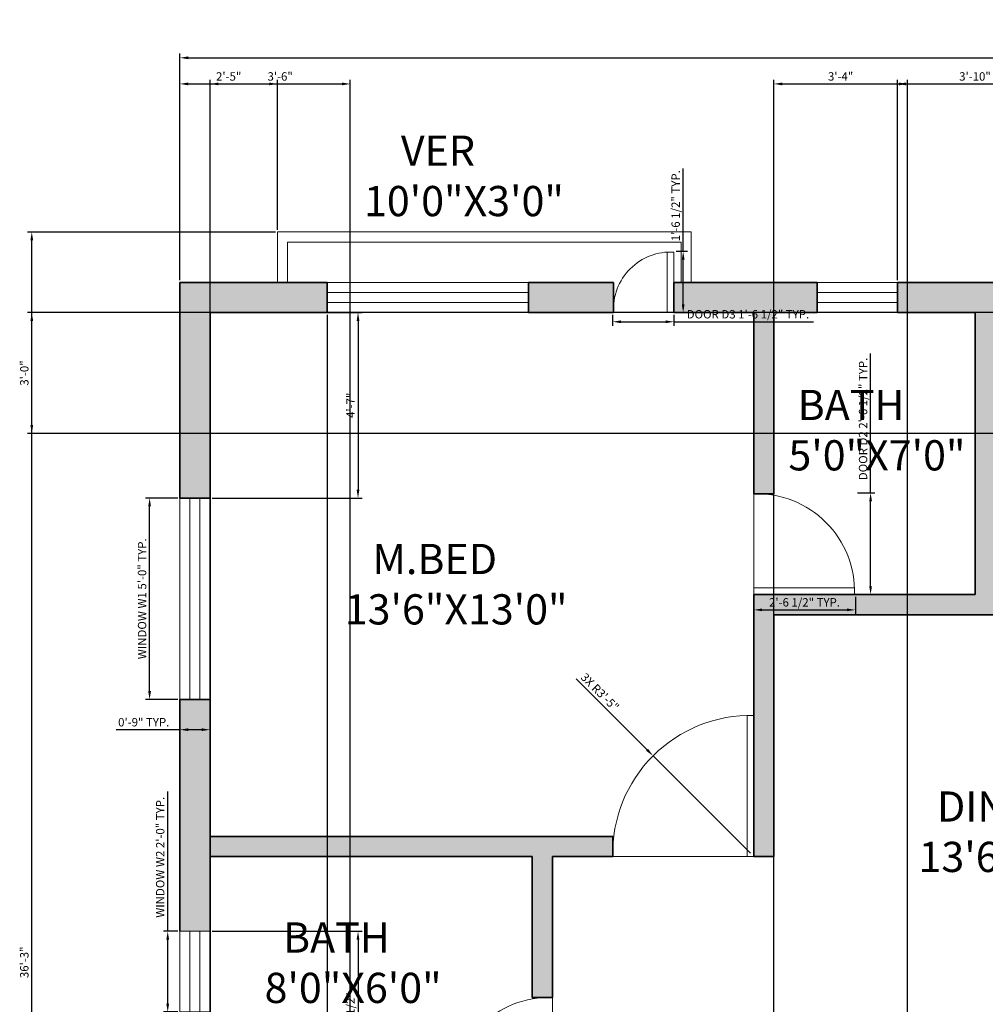
# Model space of a CAD drawing. Units: inches. Extents: x 1851 to 3979, y 3948 to 8145.
# Tile 2 of 4: x 1851 to 2139, y 4198 to 4491. Entities that reach past the tile are written whole.
import ezdxf

# ---------------------------------------------------------------- set-up
doc = ezdxf.new("R2010")
doc.units = ezdxf.units.IN
for name, color, linetype, lineweight in [('A-ANNO-DIMS', 2, 'Continuous', 18), ('A-GLAZ', 140, 'Continuous', 18), ('A-WALL', 7, 'Continuous', 35)]:
    doc.layers.add(name, color=color, linetype=linetype, lineweight=lineweight)
for name, color, linetype, lineweight, true_color in [('A-AREA-IDEN', 9, 'Continuous', 18, 0xc7c8ca), ('A-DOOR', 52, 'Continuous', 18, 0xc8c92d), ('A-FLOR-RAIL', 52, 'Continuous', 18, 0xc8c92d), ('A-WALL-PATT', 159, 'Continuous', 13, 0x22346e)]:
    doc.layers.add(name, color=color, linetype=linetype, lineweight=lineweight, true_color=true_color)
doc.styles.get("Standard").update_dxf_attribs({"font": 'arial.ttf'})
doc.dimstyles.new('ISO-25', dxfattribs={"dimtxt": 2.5, "dimasz": 2.5, "dimexe": 1.25, "dimexo": 0.625, "dimtad": 1, "dimlunit": 3, "dimtxsty": 'Standard', "dimcen": 2.5, "dimadec": 0, "dimazin": 0, "dimtfac": 1, "dimtmove": 0, "dimatfit": 3, "dimfxl": 1, "dimarcsym": 0})

# ---------------------------------------------------------------- blocks, each defined once
blk = doc.blocks.new('*D1')
at = {"layer": 'A-ANNO-DIMS', "color": 0, "lineweight": -2, "transparency": 16777216}
for p, q in [((1898.74, 4438.02), (1898.74, 4480.98)), ((2677.74, 4438.02), (2677.74, 4480.98)), ((1901.24, 4479.73), (2675.24, 4479.73))]:
    blk.add_line(p, q, dxfattribs=at)
at = {"layer": 'A-ANNO-DIMS', "color": 0, "transparency": 16777216}
for points in [[(1901.24, 4480.15), (1901.24, 4479.31), (1898.74, 4479.73)], [(2675.24, 4480.15), (2675.24, 4479.31), (2677.74, 4479.73)]]:
    blk.add_solid(points, dxfattribs=at)
at = {"layer": 'Defpoints', "color": 0, "transparency": 16777216}
for p in [(2677.74, 4479.73), (1898.74, 4437.39), (2677.74, 4437.39)]:
    blk.add_point(p, dxfattribs=at)
at = {"layer": 'A-ANNO-DIMS', "color": 0, "transparency": 16777216, "insert": (2288.24, 4484.95), "char_height": 9, "attachment_point": 5}
blk.add_mtext('64\'-11"', dxfattribs=at)
blk = doc.blocks.new('DOOR-SINGLE-42IN')
for p, q in [((42, 42), (40, 42)), ((40, 42), (40, 0)), ((42, 0), (42, 42)), ((40, 0), (42, 0))]:
    blk.add_line(p, q)
blk.add_arc((41, 1), 41.01, 88.6028, 181.3972)
blk = doc.blocks.new('DOOR-SINGLE-30IN')
for p, q in [((30, 2), (0, 2)), ((0, 2), (0, 0)), ((0, 0), (30, 0)), ((30, 0), (30, 2))]:
    blk.add_line(p, q)
blk.add_arc((1, 1), 29.02, 358.0251, 91.9749)
blk = doc.blocks.new('DOOR-SINGLE-18IN')
for p, q in [((18, 18), (16, 18)), ((16, 18), (16, 0)), ((18, 0), (18, 18)), ((16, 0), (18, 0))]:
    blk.add_line(p, q)
blk.add_arc((17, 1), 17.03, 86.6335, 183.3665)
blk = doc.blocks.new('WINDOW-60IN')
for p, q in [((0, 9), (60, 9)), ((0, 0), (0, 9)), ((60, 9), (60, 0)), ((0, 6), (60, 6)), ((0, 3), (60, 3)), ((60, 0), (0, 0))]:
    blk.add_line(p, q)
blk = doc.blocks.new('WINDOW-24IN')
for p, q in [((0, 0), (0, 9)), ((0, 9), (24, 9)), ((24, 9), (24, 0)), ((0, 6), (24, 6)), ((0, 3), (24, 3)), ((24, 0), (0, 0))]:
    blk.add_line(p, q)
blk = doc.blocks.new('*D10')
at = {"layer": 'A-ANNO-DIMS', "color": 0, "lineweight": -2, "transparency": 16777216}
for p, q in [((1898.11, 4348.62), (1888.49, 4348.62)), ((1889.74, 4291.12), (1889.74, 4346.12)), ((1898.11, 4288.62), (1888.49, 4288.62))]:
    blk.add_line(p, q, dxfattribs=at)
at = {"layer": 'A-ANNO-DIMS', "color": 0, "transparency": 16777216}
for points in [[(1889.32, 4346.12), (1890.15, 4346.12), (1889.74, 4348.62)], [(1889.32, 4291.12), (1890.15, 4291.12), (1889.74, 4288.62)]]:
    blk.add_solid(points, dxfattribs=at)
at = {"layer": 'Defpoints', "color": 0, "transparency": 16777216}
for p in [(1889.74, 4348.62), (1898.74, 4348.62), (1898.74, 4288.62)]:
    blk.add_point(p, dxfattribs=at)
at = {"layer": 'A-ANNO-DIMS', "color": 0, "transparency": 16777216, "insert": (1887.82, 4318.62), "char_height": 2.5, "attachment_point": 5, "rotation": 90}
blk.add_mtext('WINDOW W1 5\'-0" TYP.', dxfattribs=at)
blk = doc.blocks.new('*D11')
at = {"layer": 'A-ANNO-DIMS', "color": 0, "lineweight": -2, "transparency": 16777216}
for p, q in [((1898.74, 4288), (1898.74, 4278.37)), ((1907.74, 4288), (1907.74, 4278.37)), ((1898.74, 4279.62), (1879.75, 4279.62)), ((1905.24, 4279.62), (1901.24, 4279.62))]:
    blk.add_line(p, q, dxfattribs=at)
at = {"layer": 'A-ANNO-DIMS', "color": 0, "transparency": 16777216}
for points in [[(1901.24, 4280.04), (1901.24, 4279.21), (1898.74, 4279.62)], [(1905.24, 4280.04), (1905.24, 4279.21), (1907.74, 4279.62)]]:
    blk.add_solid(points, dxfattribs=at)
at = {"layer": 'Defpoints', "color": 0, "transparency": 16777216}
for p in [(1898.74, 4288.62), (1907.74, 4288.62), (1898.74, 4279.62)]:
    blk.add_point(p, dxfattribs=at)
at = {"layer": 'A-ANNO-DIMS', "color": 0, "transparency": 16777216, "insert": (1887.99, 4281.53), "char_height": 2.5, "attachment_point": 5}
blk.add_mtext('0\'-9" TYP.', dxfattribs=at)
blk = doc.blocks.new('*D12')
at = {"layer": 'A-ANNO-DIMS', "color": 0, "lineweight": -2, "transparency": 16777216}
for p, q in [((1895.14, 4219.57), (1895.14, 4261.17)), ((1898.11, 4219.57), (1893.89, 4219.57)), ((1895.14, 4198.07), (1895.14, 4217.07)), ((1898.11, 4195.57), (1893.89, 4195.57))]:
    blk.add_line(p, q, dxfattribs=at)
at = {"layer": 'A-ANNO-DIMS', "color": 0, "transparency": 16777216}
for points in [[(1894.72, 4217.07), (1895.55, 4217.07), (1895.14, 4219.57)], [(1894.72, 4198.07), (1895.55, 4198.07), (1895.14, 4195.57)]]:
    blk.add_solid(points, dxfattribs=at)
at = {"layer": 'Defpoints', "color": 0, "transparency": 16777216}
for p in [(1895.14, 4219.57), (1898.74, 4219.57), (1898.74, 4195.57)]:
    blk.add_point(p, dxfattribs=at)
at = {"layer": 'A-ANNO-DIMS', "color": 0, "transparency": 16777216, "insert": (1893.22, 4241.62), "char_height": 2.5, "attachment_point": 5, "rotation": 90}
blk.add_mtext('WINDOW W2 2\'-0" TYP.', dxfattribs=at)
blk = doc.blocks.new('*D20')
at = {"layer": 'A-ANNO-DIMS', "color": 0, "lineweight": -2, "transparency": 16777216}
for p, q in [((2104.55, 4350.13), (2104.55, 4391.7)), ((2100.64, 4350.13), (2105.8, 4350.13)), ((2104.55, 4322.35), (2104.55, 4347.63)), ((2100.64, 4319.85), (2105.8, 4319.85))]:
    blk.add_line(p, q, dxfattribs=at)
at = {"layer": 'A-ANNO-DIMS', "color": 0, "transparency": 16777216}
for points in [[(2104.14, 4347.63), (2104.97, 4347.63), (2104.55, 4350.13)], [(2104.14, 4322.35), (2104.97, 4322.35), (2104.55, 4319.85)]]:
    blk.add_solid(points, dxfattribs=at)
at = {"layer": 'Defpoints', "color": 0, "transparency": 16777216}
for p in [(2100.01, 4350.13), (2104.55, 4350.13), (2100.01, 4319.85)]:
    blk.add_point(p, dxfattribs=at)
at = {"layer": 'A-ANNO-DIMS', "color": 0, "transparency": 16777216, "insert": (2102.64, 4372.17), "char_height": 2.5, "attachment_point": 5, "rotation": 90}
blk.add_mtext('DOOR D2 2\'-6 1/2" TYP.', dxfattribs=at)
blk = doc.blocks.new('*D21')
at = {"layer": 'A-ANNO-DIMS', "color": 0, "lineweight": -2, "transparency": 16777216}
for p, q in [((2069.74, 4319.23), (2069.74, 4314.06)), ((2100.01, 4319.23), (2100.01, 4314.06)), ((2072.24, 4315.31), (2097.51, 4315.31))]:
    blk.add_line(p, q, dxfattribs=at)
at = {"layer": 'A-ANNO-DIMS', "color": 0, "transparency": 16777216}
for points in [[(2072.24, 4315.73), (2072.24, 4314.9), (2069.74, 4315.31)], [(2097.51, 4315.73), (2097.51, 4314.9), (2100.01, 4315.31)]]:
    blk.add_solid(points, dxfattribs=at)
at = {"layer": 'Defpoints', "color": 0, "transparency": 16777216}
for p in [(2069.74, 4319.85), (2100.01, 4319.85), (2100.01, 4315.31)]:
    blk.add_point(p, dxfattribs=at)
at = {"layer": 'A-ANNO-DIMS', "color": 0, "transparency": 16777216, "insert": (2084.87, 4317.23), "char_height": 2.5, "attachment_point": 5}
blk.add_mtext('2\'-6 1/2" TYP.', dxfattribs=at)
blk = doc.blocks.new('*D22')
at = {"layer": 'A-ANNO-DIMS', "color": 0, "lineweight": -2, "transparency": 16777216}
for p, q in [((2027.68, 4403.23), (2027.68, 4399.86)), ((2045.97, 4403.23), (2045.97, 4399.86)), ((2030.18, 4401.11), (2043.47, 4401.11)), ((2045.97, 4401.11), (2087.54, 4401.11))]:
    blk.add_line(p, q, dxfattribs=at)
at = {"layer": 'A-ANNO-DIMS', "color": 0, "transparency": 16777216}
for points in [[(2030.18, 4401.53), (2030.18, 4400.7), (2027.68, 4401.11)], [(2043.47, 4401.53), (2043.47, 4400.7), (2045.97, 4401.11)]]:
    blk.add_solid(points, dxfattribs=at)
at = {"layer": 'Defpoints', "color": 0, "transparency": 16777216}
for p in [(2027.68, 4403.85), (2045.97, 4403.85), (2045.97, 4401.11)]:
    blk.add_point(p, dxfattribs=at)
at = {"layer": 'A-ANNO-DIMS', "color": 0, "transparency": 16777216, "insert": (2068.01, 4403.03), "char_height": 2.5, "attachment_point": 5}
blk.add_mtext('DOOR D3 1\'-6 1/2" TYP.', dxfattribs=at)
blk = doc.blocks.new('*D23')
at = {"layer": 'A-ANNO-DIMS', "color": 0, "lineweight": -2, "transparency": 16777216}
for p, q in [((2048.71, 4422.14), (2048.71, 4446.72)), ((2046.59, 4422.14), (2049.96, 4422.14)), ((2048.71, 4406.35), (2048.71, 4419.64)), ((2046.59, 4403.85), (2049.96, 4403.85))]:
    blk.add_line(p, q, dxfattribs=at)
at = {"layer": 'A-ANNO-DIMS', "color": 0, "transparency": 16777216}
for points in [[(2048.3, 4419.64), (2049.13, 4419.64), (2048.71, 4422.14)], [(2048.3, 4406.35), (2049.13, 4406.35), (2048.71, 4403.85)]]:
    blk.add_solid(points, dxfattribs=at)
at = {"layer": 'Defpoints', "color": 0, "transparency": 16777216}
for p in [(2045.97, 4422.14), (2048.71, 4422.14), (2045.97, 4403.85)]:
    blk.add_point(p, dxfattribs=at)
at = {"layer": 'A-ANNO-DIMS', "color": 0, "transparency": 16777216, "insert": (2046.8, 4435.68), "char_height": 2.5, "attachment_point": 5, "rotation": 90}
blk.add_mtext('1\'-6 1/2" TYP.', dxfattribs=at)
blk = doc.blocks.new('*D27')
at = {"layer": 'A-ANNO-DIMS', "color": 0, "lineweight": -2, "transparency": 16777216}
for p, q in [((1907.74, 4002.48), (1907.74, 4473.2)), ((1949.54, 4002.48), (1949.54, 4473.2)), ((1910.24, 4471.95), (1947.04, 4471.95))]:
    blk.add_line(p, q, dxfattribs=at)
at = {"layer": 'A-ANNO-DIMS', "color": 0, "transparency": 16777216}
for points in [[(1910.24, 4472.37), (1910.24, 4471.54), (1907.74, 4471.95)], [(1947.04, 4472.37), (1947.04, 4471.54), (1949.54, 4471.95)]]:
    blk.add_solid(points, dxfattribs=at)
at = {"layer": 'Defpoints', "color": 0, "transparency": 16777216}
for p in [(1949.54, 4471.95), (1907.74, 4001.85), (1949.54, 4001.85)]:
    blk.add_point(p, dxfattribs=at)
at = {"layer": 'A-ANNO-DIMS', "color": 0, "transparency": 16777216, "insert": (1928.64, 4473.86), "char_height": 2.5, "attachment_point": 5}
blk.add_mtext('3\'-6"', dxfattribs=at)
blk = doc.blocks.new('*D28')
at = {"layer": 'A-ANNO-DIMS', "color": 0, "lineweight": -2, "transparency": 16777216}
for p, q in [((2075.74, 4002.48), (2075.74, 4473.2)), ((2115.51, 4002.48), (2115.51, 4473.2)), ((2078.24, 4471.95), (2113.01, 4471.95))]:
    blk.add_line(p, q, dxfattribs=at)
at = {"layer": 'A-ANNO-DIMS', "color": 0, "transparency": 16777216}
for points in [[(2078.24, 4472.37), (2078.24, 4471.54), (2075.74, 4471.95)], [(2113.01, 4472.37), (2113.01, 4471.54), (2115.51, 4471.95)]]:
    blk.add_solid(points, dxfattribs=at)
at = {"layer": 'Defpoints', "color": 0, "transparency": 16777216}
for p in [(2115.51, 4471.95), (2075.74, 4001.85), (2115.51, 4001.85)]:
    blk.add_point(p, dxfattribs=at)
at = {"layer": 'A-ANNO-DIMS', "color": 0, "transparency": 16777216, "insert": (2095.62, 4473.86), "char_height": 2.5, "attachment_point": 5}
blk.add_mtext('3\'-4"', dxfattribs=at)
blk = doc.blocks.new('*D31')
at = {"layer": 'A-ANNO-DIMS', "color": 0, "lineweight": -2, "transparency": 16777216}
for p, q in [((1898.74, 4413.48), (1898.74, 4473.2)), ((1927.87, 4428.48), (1927.87, 4473.2)), ((1901.24, 4471.95), (1925.37, 4471.95))]:
    blk.add_line(p, q, dxfattribs=at)
at = {"layer": 'A-ANNO-DIMS', "color": 0, "transparency": 16777216}
for points in [[(1901.24, 4472.37), (1901.24, 4471.54), (1898.74, 4471.95)], [(1925.37, 4472.37), (1925.37, 4471.54), (1927.87, 4471.95)]]:
    blk.add_solid(points, dxfattribs=at)
at = {"layer": 'Defpoints', "color": 0, "transparency": 16777216}
for p in [(1927.87, 4471.95), (1927.87, 4427.85), (1898.74, 4412.85)]:
    blk.add_point(p, dxfattribs=at)
at = {"layer": 'A-ANNO-DIMS', "color": 0, "transparency": 16777216, "insert": (1913.3, 4473.86), "char_height": 2.5, "attachment_point": 5}
blk.add_mtext('2\'-5"', dxfattribs=at)
blk = doc.blocks.new('*D35')
at = {"layer": 'A-ANNO-DIMS', "color": 0, "lineweight": -2, "transparency": 16777216}
for p, q in [((2331.11, 4403.85), (1853.39, 4403.85)), ((1854.64, 4370.35), (1854.64, 4401.35)), ((2331.11, 4367.85), (1853.39, 4367.85))]:
    blk.add_line(p, q, dxfattribs=at)
at = {"layer": 'A-ANNO-DIMS', "color": 0, "transparency": 16777216}
for points in [[(1854.22, 4401.35), (1855.05, 4401.35), (1854.64, 4403.85)], [(1854.22, 4370.35), (1855.05, 4370.35), (1854.64, 4367.85)]]:
    blk.add_solid(points, dxfattribs=at)
at = {"layer": 'Defpoints', "color": 0, "transparency": 16777216}
for p in [(1854.64, 4403.85), (2331.74, 4403.85), (2331.74, 4367.85)]:
    blk.add_point(p, dxfattribs=at)
at = {"layer": 'A-ANNO-DIMS', "color": 0, "transparency": 16777216, "insert": (1852.73, 4385.85), "char_height": 2.5, "attachment_point": 5, "rotation": 90}
blk.add_mtext('3\'-0"', dxfattribs=at)
blk = doc.blocks.new('*D37')
at = {"layer": 'A-ANNO-DIMS', "color": 0, "lineweight": -2, "transparency": 16777216}
for p, q in [((1908.36, 4219.57), (1953.09, 4219.57)), ((1951.84, 4217.07), (1951.84, 4172.35)), ((1908.36, 4169.85), (1953.09, 4169.85))]:
    blk.add_line(p, q, dxfattribs=at)
at = {"layer": 'A-ANNO-DIMS', "color": 0, "transparency": 16777216}
for points in [[(1951.42, 4217.07), (1952.25, 4217.07), (1951.84, 4219.57)], [(1951.42, 4172.35), (1952.25, 4172.35), (1951.84, 4169.85)]]:
    blk.add_solid(points, dxfattribs=at)
at = {"layer": 'Defpoints', "color": 0, "transparency": 16777216}
for p in [(1907.74, 4219.57), (1907.74, 4169.85), (1951.84, 4169.85)]:
    blk.add_point(p, dxfattribs=at)
at = {"layer": 'A-ANNO-DIMS', "color": 0, "transparency": 16777216, "insert": (1949.92, 4194.71), "char_height": 2.5, "attachment_point": 5, "rotation": 90}
blk.add_mtext('4\'-1 1/2"', dxfattribs=at)
blk = doc.blocks.new('*D38')
at = {"layer": 'A-ANNO-DIMS', "color": 0, "lineweight": -2, "transparency": 16777216}
for p, q in [((1908.36, 4403.85), (1953.09, 4403.85)), ((1951.84, 4401.35), (1951.84, 4351.12)), ((1908.36, 4348.62), (1953.09, 4348.62))]:
    blk.add_line(p, q, dxfattribs=at)
at = {"layer": 'A-ANNO-DIMS', "color": 0, "transparency": 16777216}
for points in [[(1951.42, 4401.35), (1952.25, 4401.35), (1951.84, 4403.85)], [(1951.42, 4351.12), (1952.25, 4351.12), (1951.84, 4348.62)]]:
    blk.add_solid(points, dxfattribs=at)
at = {"layer": 'Defpoints', "color": 0, "transparency": 16777216}
for p in [(1907.74, 4403.85), (1907.74, 4348.62), (1951.84, 4348.62)]:
    blk.add_point(p, dxfattribs=at)
at = {"layer": 'A-ANNO-DIMS', "color": 0, "transparency": 16777216, "insert": (1949.96, 4376.24), "char_height": 2.5, "attachment_point": 5, "rotation": 90}
blk.add_mtext('4\'-7"', dxfattribs=at)
blk = doc.blocks.new('*D39')
at = {"layer": 'A-ANNO-DIMS', "color": 0, "lineweight": -2, "transparency": 16777216}
for p, q in [((1927.24, 4427.85), (1853.39, 4427.85)), ((1854.64, 3995.35), (1854.64, 4425.35)), ((1898.11, 3992.85), (1853.39, 3992.85))]:
    blk.add_line(p, q, dxfattribs=at)
at = {"layer": 'A-ANNO-DIMS', "color": 0, "transparency": 16777216}
for points in [[(1854.22, 4425.35), (1855.05, 4425.35), (1854.64, 4427.85)], [(1854.22, 3995.35), (1855.05, 3995.35), (1854.64, 3992.85)]]:
    blk.add_solid(points, dxfattribs=at)
at = {"layer": 'Defpoints', "color": 0, "transparency": 16777216}
for p in [(1854.64, 4427.85), (1927.87, 4427.85), (1898.74, 3992.85)]:
    blk.add_point(p, dxfattribs=at)
at = {"layer": 'A-ANNO-DIMS', "color": 0, "transparency": 16777216, "insert": (1852.73, 4210.35), "char_height": 2.5, "attachment_point": 5, "rotation": 90}
blk.add_mtext('36\'-3"', dxfattribs=at)
blk = doc.blocks.new('*D46')
at = {"layer": 'A-ANNO-DIMS', "color": 0, "lineweight": -2, "transparency": 16777216}
for p, q in [((1907.74, 4403.23), (1907.74, 3947.5)), ((1942.66, 4403.23), (1942.66, 3947.5)), ((1910.24, 3948.75), (1940.16, 3948.75))]:
    blk.add_line(p, q, dxfattribs=at)
at = {"layer": 'A-ANNO-DIMS', "color": 0, "transparency": 16777216}
for points in [[(1910.24, 3949.17), (1910.24, 3948.34), (1907.74, 3948.75)], [(1940.16, 3949.17), (1940.16, 3948.34), (1942.66, 3948.75)]]:
    blk.add_solid(points, dxfattribs=at)
at = {"layer": 'Defpoints', "color": 0, "transparency": 16777216}
for p in [(1907.74, 4403.85), (1942.66, 4403.85), (1942.66, 3948.75)]:
    blk.add_point(p, dxfattribs=at)
at = {"layer": 'A-ANNO-DIMS', "color": 0, "transparency": 16777216, "insert": (1925.2, 3950.64), "char_height": 2.5, "attachment_point": 5}
blk.add_mtext('2\'-11"', dxfattribs=at)
blk = doc.blocks.new('*D49')
at = {"layer": 'A-ANNO-DIMS', "color": 0, "lineweight": -2, "transparency": 16777216}
for p, q in [((2112.59, 4413.48), (2112.59, 4473.2)), ((2158.72, 4413.48), (2158.72, 4473.2)), ((2115.09, 4471.95), (2156.22, 4471.95))]:
    blk.add_line(p, q, dxfattribs=at)
at = {"layer": 'A-ANNO-DIMS', "color": 0, "transparency": 16777216}
for points in [[(2115.09, 4472.37), (2115.09, 4471.54), (2112.59, 4471.95)], [(2156.22, 4472.37), (2156.22, 4471.54), (2158.72, 4471.95)]]:
    blk.add_solid(points, dxfattribs=at)
at = {"layer": 'Defpoints', "color": 0, "transparency": 16777216}
for p in [(2158.72, 4471.95), (2112.59, 4412.85), (2158.72, 4412.85)]:
    blk.add_point(p, dxfattribs=at)
at = {"layer": 'A-ANNO-DIMS', "color": 0, "transparency": 16777216, "insert": (2135.66, 4473.86), "char_height": 2.5, "attachment_point": 5}
blk.add_mtext('3\'-10"', dxfattribs=at)
blk = doc.blocks.new('*D53')
at = {"layer": 'A-ANNO-DIMS', "color": 0, "lineweight": -2, "transparency": 16777216}
for p, q in [((2016.8, 4294.79), (2037.97, 4273.62)), ((2068.74, 4242.85), (2039.74, 4271.85))]:
    blk.add_line(p, q, dxfattribs=at)
at = {"layer": 'A-ANNO-DIMS', "color": 0, "transparency": 16777216}
blk.add_solid([(2038.26, 4273.92), (2037.67, 4273.33), (2039.74, 4271.85)], dxfattribs=at)
at = {"layer": 'Defpoints', "color": 0, "transparency": 16777216}
for p in [(2039.74, 4271.85), (2068.74, 4242.85)]:
    blk.add_point(p, dxfattribs=at)
at = {"layer": 'A-ANNO-DIMS', "color": 0, "transparency": 16777216, "insert": (2023.68, 4290.6), "char_height": 2.5, "attachment_point": 5, "rotation": 315}
blk.add_mtext('3X R3\'-5"', dxfattribs=at)

msp = doc.modelspace()

# ---------------------------------------------------------------- hatches: boundary and pattern name
at = {"layer": 'A-WALL-PATT'}
h = msp.add_hatch(dxfattribs=at)
h.set_pattern_fill('GRASS', color=256, scale=3)
h.paths.add_polyline_path([(1942.655, 4412.855), (1898.736, 4412.855), (1898.736, 4348.625), (1907.736, 4348.625), (1907.736, 4403.855), (1942.655, 4403.855)])
h.paths.add_polyline_path([(2027.97, 4412.855), (2002.655, 4412.855), (2002.655, 4403.855), (2027.97, 4403.855, -0.0293864), (2027.97, 4405.855)])
h.paths.add_polyline_path([(2088.59, 4412.855), (2045.97, 4412.855), (2045.97, 4403.855), (2069.736, 4403.855), (2069.736, 4349.855, -0.0172363), (2071.736, 4349.855), (2075.736, 4349.855), (2075.736, 4403.855), (2088.59, 4403.855)])
h.paths.add_polyline_path([(2158.724, 4412.855), (2112.59, 4412.855), (2112.59, 4403.855), (2135.736, 4403.855), (2135.736, 4319.855), (2069.736, 4319.855), (2069.736, 4241.855), (2075.736, 4241.855), (2075.736, 4313.855), (2141.736, 4313.855), (2141.736, 4403.855), (2158.724, 4403.855)])
h.paths.add_polyline_path([(2244.736, 4403.855), (2256.687, 4403.855), (2256.687, 4412.855), (2218.724, 4412.855), (2218.724, 4403.855), (2238.736, 4403.855), (2238.736, 4319.855), (2171.736, 4319.855), (2171.736, 4315.855, -0.0172363), (2171.736, 4313.855), (2238.736, 4313.855), (2238.736, 4211.855), (2242.736, 4211.855, -0.0121933), (2244.736, 4211.855)])
h.paths.add_polyline_path([(2356.912, 4412.855), (2353.884, 4412.855), (2312.372, 4412.855), (2312.372, 4403.855), (2331.736, 4403.855), (2331.736, 4211.855, -0.0121933), (2333.736, 4211.855), (2337.736, 4211.855), (2337.736, 4313.855), (2404.736, 4313.855, -0.0172363), (2404.736, 4315.855), (2404.736, 4319.855), (2337.736, 4319.855), (2337.736, 4403.855), (2353.884, 4403.855), (2356.912, 4403.855)])
h.paths.add_polyline_path([(2440.736, 4403.855), (2451.168, 4403.855), (2451.168, 4412.855), (2401.884, 4412.855), (2401.884, 4403.855), (2434.736, 4403.855), (2434.736, 4313.855), (2500.736, 4313.855), (2500.736, 4241.855), (2506.736, 4241.855), (2506.736, 4283.855), (2506.736, 4319.855), (2476.736, 4319.855), (2440.736, 4319.855)])
h.paths.add_polyline_path([(2506.736, 4403.855), (2516.983, 4403.855), (2516.983, 4412.855), (2475.168, 4412.855), (2475.168, 4403.855), (2500.736, 4403.855), (2500.736, 4349.855), (2504.736, 4349.855, -0.0172363), (2506.736, 4349.855)])
h.paths.add_polyline_path([(2544.739, 4412.855), (2534.983, 4412.855), (2534.983, 4405.855, -0.0293864), (2534.983, 4403.855), (2544.739, 4403.855)])
h.paths.add_polyline_path([(2677.736, 4412.855), (2618.736, 4412.855), (2616.739, 4412.855), (2616.739, 4403.855), (2668.736, 4403.855), (2668.736, 4349.414), (2677.736, 4349.414), (2677.736, 4403.855)])
h.paths.add_polyline_path([(2677.736, 4301.414), (2668.736, 4301.414), (2668.736, 4247.855), (2548.736, 4247.855), (2548.736, 4243.855, -0.0121933), (2548.736, 4241.855), (2572.736, 4241.855), (2572.736, 4187.855, -0.0293864), (2574.736, 4187.855), (2578.736, 4187.855), (2578.736, 4241.855), (2668.736, 4241.855), (2668.736, 4216.247), (2677.736, 4216.247)])
h.paths.add_polyline_path([(2677.736, 4192.247), (2668.736, 4192.247), (2668.736, 4169.855), (2572.736, 4169.855), (2548.736, 4169.855, -0.0424267), (2549.319, 4163.855), (2572.736, 4163.855), (2668.736, 4163.855), (2668.736, 4130.251), (2677.736, 4130.251)])
h.paths.add_polyline_path([(2677.736, 4001.855), (2677.736, 4058.251), (2668.736, 4058.251), (2668.736, 4001.855), (2614.828, 4001.855), (2614.828, 3992.855), (2618.736, 3992.855), (2677.736, 3992.855)])
h.paths.add_polyline_path([(2554.828, 4001.855), (2512.736, 4001.855), (2512.736, 4163.855), (2512.736, 4169.855), (2506.736, 4169.855), (2506.736, 4127.855), (2506.736, 4001.855), (2470.736, 4001.855), (2470.736, 3992.855), (2554.828, 3992.855)])
h.paths.add_polyline_path([(2410.736, 4001.855), (2337.736, 4001.855), (2337.736, 3992.855), (2410.736, 3992.855)])
h.paths.add_polyline_path([(2337.736, 4169.855), (2331.736, 4169.855), (2331.736, 4075.855), (2337.736, 4075.855)])
h.paths.add_polyline_path([(2464.736, 4167.855, -0.0121933), (2464.736, 4169.855), (2337.736, 4169.855), (2337.736, 4163.855), (2464.736, 4163.855)])
h.paths.add_polyline_path([(2244.736, 4169.855), (2202.736, 4169.855), (2117.736, 4169.855, -0.0121933), (2117.736, 4167.855), (2117.736, 4163.855), (2238.736, 4163.855), (2238.736, 4075.855), (2244.736, 4075.855)])
h.paths.add_polyline_path([(2325.736, 4001.855), (2250.736, 4001.855), (2250.736, 3992.855), (2325.736, 3992.855)])
h.paths.add_polyline_path([(2238.736, 4001.855), (2175.511, 4001.855), (2175.511, 3992.855), (2238.736, 3992.855)])
h.paths.add_polyline_path([(2115.511, 4001.855), (2075.736, 4001.855), (2075.736, 4169.855), (2069.736, 4169.855), (2069.736, 4127.855), (2069.736, 4001.855), (2009.539, 4001.855), (2009.539, 3992.855), (2115.511, 3992.855)])
h.paths.add_polyline_path([(1949.539, 4001.855), (1907.736, 4001.855), (1907.736, 4049.088), (1898.736, 4049.088), (1898.736, 3992.855), (1949.539, 3992.855)])
h.paths.add_polyline_path([(1907.736, 4163.855), (2027.736, 4163.855), (2027.736, 4167.855, -0.0121933), (2027.736, 4169.855), (1907.736, 4169.855), (1907.736, 4195.575), (1898.736, 4195.575), (1898.736, 4109.088), (1907.736, 4109.088)])
h.paths.add_polyline_path([(2027.736, 4247.855), (1907.736, 4247.855), (1907.736, 4288.625), (1898.736, 4288.625), (1898.736, 4219.575), (1907.736, 4219.575), (1907.736, 4241.855), (2003.736, 4241.855), (2003.736, 4219.575), (2003.736, 4199.855), (2007.736, 4199.855, -0.0172363), (2009.736, 4199.855), (2009.736, 4241.855), (2027.736, 4241.855, -0.0121933), (2027.736, 4243.855)])
h = msp.add_hatch(dxfattribs=at)
h.set_pattern_fill('GRASS', color=256, scale=3)
h.paths.add_polyline_path([(1942.655, 4412.855), (1898.736, 4412.855), (1898.736, 4348.625), (1907.736, 4348.625), (1907.736, 4403.855), (1942.655, 4403.855)])
h.paths.add_polyline_path([(2027.97, 4412.855), (2002.655, 4412.855), (2002.655, 4403.855), (2027.97, 4403.855, -0.0293864), (2027.97, 4405.855)])
h.paths.add_polyline_path([(2088.59, 4412.855), (2045.97, 4412.855), (2045.97, 4403.855), (2069.736, 4403.855), (2069.736, 4349.855, -0.0172363), (2071.736, 4349.855), (2075.736, 4349.855), (2075.736, 4403.855), (2088.59, 4403.855)])
h.paths.add_polyline_path([(2158.724, 4412.855), (2112.59, 4412.855), (2112.59, 4403.855), (2135.736, 4403.855), (2135.736, 4319.855), (2069.736, 4319.855), (2069.736, 4241.855), (2075.736, 4241.855), (2075.736, 4313.855), (2141.736, 4313.855), (2141.736, 4343.855), (2141.736, 4403.855), (2158.724, 4403.855)])
h.paths.add_polyline_path([(2256.687, 4412.855), (2218.724, 4412.855), (2218.724, 4403.855), (2238.736, 4403.855), (2238.736, 4319.855), (2171.736, 4319.855), (2171.736, 4315.855, -0.0172363), (2171.736, 4313.855), (2238.736, 4313.855), (2238.736, 4211.855), (2242.736, 4211.855, -0.0121933), (2244.736, 4211.855), (2244.736, 4403.855), (2256.687, 4403.855)])
h.paths.add_polyline_path([(2356.912, 4412.855), (2353.884, 4412.855), (2312.372, 4412.855), (2312.372, 4403.855), (2331.736, 4403.855), (2331.736, 4211.855, -0.0121933), (2333.736, 4211.855), (2337.736, 4211.855), (2337.736, 4313.855), (2404.736, 4313.855, -0.0172363), (2404.736, 4315.855), (2404.736, 4319.855), (2337.736, 4319.855), (2337.736, 4403.855), (2353.884, 4403.855), (2356.912, 4403.855)])
h = msp.add_hatch(dxfattribs=at)
h.set_pattern_fill('GRASS', color=256, scale=3)
h.paths.add_polyline_path([(1907.736, 4403.855), (1942.655, 4403.855), (1942.655, 4412.855), (1898.736, 4412.855), (1898.736, 4348.625), (1907.736, 4348.625)])
h.paths.add_polyline_path([(1907.736, 4288.625), (1898.736, 4288.625), (1898.736, 4219.575), (1907.736, 4219.575), (1907.736, 4241.855), (2003.736, 4241.855), (2003.736, 4219.575), (2003.736, 4199.855), (2007.736, 4199.855, -0.0172363), (2009.736, 4199.855), (2009.736, 4241.855), (2027.736, 4241.855, -0.0121933), (2027.736, 4243.855), (2027.736, 4247.855), (1907.736, 4247.855)])
h.paths.add_polyline_path([(1907.736, 4163.855), (2027.736, 4163.855), (2027.736, 4167.855, -0.0121933), (2027.736, 4169.855), (1907.736, 4169.855), (1907.736, 4195.575), (1898.736, 4195.575), (1898.736, 4109.088), (1907.736, 4109.088)])
h.paths.add_polyline_path([(1907.736, 4049.088), (1898.736, 4049.088), (1898.736, 3992.855), (1949.539, 3992.855), (1949.539, 4001.855), (1907.736, 4001.855)])
h = msp.add_hatch(color=256, dxfattribs=at)
h.dxf.hatch_style = 1
h.paths.add_polyline_path([(1907.736, 4163.855), (2027.736, 4163.855), (2027.736, 4167.855, -0.0121933), (2027.736, 4169.855), (1907.736, 4169.855), (1907.736, 4195.575), (1898.736, 4195.575), (1898.736, 4109.088), (1907.736, 4109.088)])
h.paths.add_polyline_path([(1907.736, 4049.088), (1898.736, 4049.088), (1898.736, 3992.855), (1949.539, 3992.855), (1949.539, 4001.855), (1907.736, 4001.855)])
h.paths.add_polyline_path([(2115.511, 4001.855), (2075.736, 4001.855), (2075.736, 4169.855), (2069.736, 4169.855), (2069.736, 4127.855), (2069.736, 4001.855), (2009.539, 4001.855), (2009.539, 3992.855), (2115.511, 3992.855)])
h.paths.add_polyline_path([(2238.736, 4001.855), (2175.511, 4001.855), (2175.511, 3992.855), (2238.736, 3992.855)])
h.paths.add_polyline_path([(2325.736, 4001.855), (2250.736, 4001.855), (2250.736, 3992.855), (2325.736, 3992.855)])
h.paths.add_polyline_path([(2410.736, 4001.855), (2337.736, 4001.855), (2337.736, 3992.855), (2410.736, 3992.855)])
h.paths.add_polyline_path([(2554.828, 4001.855), (2512.736, 4001.855), (2512.736, 4163.855), (2512.736, 4169.855), (2506.736, 4169.855), (2506.736, 4127.855), (2506.736, 4001.855), (2470.736, 4001.855), (2470.736, 3992.855), (2554.828, 3992.855)])
h.paths.add_polyline_path([(2677.736, 4001.855), (2677.736, 4058.251), (2668.736, 4058.251), (2668.736, 4001.855), (2614.828, 4001.855), (2614.828, 3992.855), (2618.736, 3992.855), (2677.736, 3992.855)])
h.paths.add_polyline_path([(2244.736, 4169.855), (2202.736, 4169.855), (2117.736, 4169.855, -0.0121933), (2117.736, 4167.855), (2117.736, 4163.855), (2238.736, 4163.855), (2238.736, 4075.855), (2244.736, 4075.855)])
h.paths.add_polyline_path([(2337.736, 4169.855), (2331.736, 4169.855), (2331.736, 4075.855), (2337.736, 4075.855)])
h.paths.add_polyline_path([(2337.736, 4063.855), (2331.736, 4063.855), (2331.736, 4004.855), (2337.736, 4004.855)])
h.paths.add_polyline_path([(2244.736, 4063.855), (2238.736, 4063.855), (2238.736, 4004.855), (2244.736, 4004.855)])
h.paths.add_polyline_path([(2464.736, 4167.855, -0.0121933), (2464.736, 4169.855), (2337.736, 4169.855), (2337.736, 4163.855), (2464.736, 4163.855)])
h.paths.add_polyline_path([(2337.736, 4313.855), (2404.736, 4313.855, -0.0172363), (2404.736, 4315.855), (2404.736, 4319.855), (2337.736, 4319.855), (2337.736, 4403.855), (2353.884, 4403.855), (2356.912, 4403.855), (2356.912, 4412.855), (2353.884, 4412.855), (2312.372, 4412.855), (2312.372, 4403.855), (2331.736, 4403.855), (2331.736, 4211.855, -0.0121933), (2333.736, 4211.855), (2337.736, 4211.855)])
h.paths.add_polyline_path([(2244.736, 4403.855), (2256.687, 4403.855), (2256.687, 4412.855), (2218.724, 4412.855), (2218.724, 4403.855), (2238.736, 4403.855), (2238.736, 4319.855), (2171.736, 4319.855), (2171.736, 4315.855, -0.0172363), (2171.736, 4313.855), (2238.736, 4313.855), (2238.736, 4211.855), (2242.736, 4211.855, -0.0121933), (2244.736, 4211.855)])
h.paths.add_polyline_path([(2506.736, 4283.855), (2506.736, 4319.855), (2476.736, 4319.855), (2440.736, 4319.855), (2440.736, 4403.855), (2451.168, 4403.855), (2451.168, 4412.855), (2401.884, 4412.855), (2401.884, 4403.855), (2434.736, 4403.855), (2434.736, 4313.855), (2500.736, 4313.855), (2500.736, 4241.855), (2506.736, 4241.855)])
h.paths.add_polyline_path([(2578.736, 4241.855), (2668.736, 4241.855), (2668.736, 4216.247), (2677.736, 4216.247), (2677.736, 4301.414), (2668.736, 4301.414), (2668.736, 4247.855), (2548.736, 4247.855), (2548.736, 4243.855, -0.0121933), (2548.736, 4241.855), (2572.736, 4241.855), (2572.736, 4187.855, -0.0293864), (2574.736, 4187.855), (2578.736, 4187.855)])
h.paths.add_polyline_path([(2677.736, 4192.247), (2668.736, 4192.247), (2668.736, 4169.855), (2572.736, 4169.855), (2548.736, 4169.855, -0.0424267), (2549.319, 4163.855), (2572.736, 4163.855), (2668.736, 4163.855), (2668.736, 4130.251), (2677.736, 4130.251)])
h.paths.add_polyline_path([(2506.736, 4403.855), (2516.983, 4403.855), (2516.983, 4412.855), (2475.168, 4412.855), (2475.168, 4403.855), (2500.736, 4403.855), (2500.736, 4349.855), (2504.736, 4349.855, -0.0172363), (2506.736, 4349.855)])
h.paths.add_polyline_path([(2677.736, 4412.855), (2618.736, 4412.855), (2616.739, 4412.855), (2616.739, 4403.855), (2668.736, 4403.855), (2668.736, 4349.414), (2677.736, 4349.414), (2677.736, 4403.855)])
h.paths.add_polyline_path([(2544.739, 4412.855), (2534.983, 4412.855), (2534.983, 4405.855, -0.0293864), (2534.983, 4403.855), (2544.739, 4403.855)])
h.paths.add_polyline_path([(2141.736, 4403.855), (2158.724, 4403.855), (2158.724, 4412.855), (2112.59, 4412.855), (2112.59, 4403.855), (2135.736, 4403.855), (2135.736, 4319.855), (2069.736, 4319.855), (2069.736, 4241.855), (2075.736, 4241.855), (2075.736, 4313.855), (2141.736, 4313.855), (2141.736, 4343.855)])
h.paths.add_polyline_path([(2075.736, 4403.855), (2088.59, 4403.855), (2088.59, 4412.855), (2045.97, 4412.855), (2045.97, 4403.855), (2069.736, 4403.855), (2069.736, 4349.855, -0.0172363), (2071.736, 4349.855), (2075.736, 4349.855)])
h.paths.add_polyline_path([(2027.97, 4412.855), (2002.655, 4412.855), (2002.655, 4403.855), (2027.97, 4403.855, -0.0293864), (2027.97, 4405.855)])
h.paths.add_polyline_path([(1942.655, 4412.855), (1898.736, 4412.855), (1898.736, 4348.625), (1907.736, 4348.625), (1907.736, 4403.855), (1942.655, 4403.855)])
h.paths.add_polyline_path([(2027.736, 4247.855), (1907.736, 4247.855), (1907.736, 4288.625), (1898.736, 4288.625), (1898.736, 4219.575), (1907.736, 4219.575), (1907.736, 4241.855), (2003.736, 4241.855), (2003.736, 4219.575), (2003.736, 4199.855), (2007.736, 4199.855, -0.0172363), (2009.736, 4199.855), (2009.736, 4241.855), (2027.736, 4241.855, -0.0121933), (2027.736, 4243.855)])

# ---------------------------------------------------------------- linework, layer by layer
at = {"layer": 'A-DOOR'}
for p, q in [((2027.97, 4403.855), (2045.97, 4403.855)), ((2069.736, 4320.855), (2069.736, 4349.855)), ((2027.736, 4241.855), (2069.736, 4241.855)), ((2009.736, 4170.855), (2009.736, 4199.855))]:
    msp.add_line(p, q, dxfattribs=at)
at = {"layer": 'A-FLOR-RAIL'}
for p, q in [((1927.869, 4424.855), (1927.869, 4427.855)), ((1927.869, 4427.855), (1930.869, 4427.855)), ((1930.869, 4427.855), (2048.075, 4427.855)), ((2048.075, 4427.855), (2051.075, 4427.855)), ((2051.075, 4427.855), (2051.075, 4424.855)), ((1927.869, 4412.855), (1927.869, 4424.855)), ((1930.869, 4424.855), (2048.075, 4424.855)), ((1930.869, 4412.855), (1930.869, 4424.855)), ((2048.075, 4424.855), (2048.075, 4412.855)), ((2051.075, 4424.855), (2051.075, 4412.855))]:
    msp.add_line(p, q, dxfattribs=at)
at = {"layer": 'A-GLAZ'}
for p, q in [((1898.736, 4288.625), (1898.736, 4348.625)), ((1898.736, 4219.575), (1907.736, 4219.575))]:
    msp.add_line(p, q, dxfattribs=at)
at = {"layer": 'A-WALL'}
for p, q in [((1898.736, 4412.855), (1942.655, 4412.855)), ((1898.736, 4348.625), (1898.736, 4412.855)), ((1942.655, 4412.855), (1942.655, 4403.855)), ((2002.655, 4412.855), (2002.655, 4403.855)), ((2002.655, 4412.855), (2027.97, 4412.855)), ((2027.97, 4412.855), (2027.97, 4403.855)), ((2045.97, 4412.855), (2045.97, 4403.855)), ((2045.97, 4412.855), (2088.59, 4412.855)), ((2088.59, 4412.855), (2088.59, 4403.855)), ((2112.59, 4412.855), (2112.59, 4403.855)), ((2112.59, 4412.855), (2158.724, 4412.855)), ((1907.736, 4403.855), (1942.655, 4403.855)), ((1907.736, 4348.625), (1907.736, 4403.855)), ((2002.655, 4403.855), (2027.97, 4403.855)), ((2045.97, 4403.855), (2069.736, 4403.855)), ((2069.736, 4349.855), (2069.736, 4403.855)), ((2075.736, 4349.855), (2075.736, 4403.855)), ((2075.736, 4403.855), (2088.59, 4403.855)), ((2112.59, 4403.855), (2135.736, 4403.855)), ((2135.736, 4319.855), (2135.736, 4403.855)), ((2069.736, 4349.855), (2075.736, 4349.855)), ((1898.736, 4348.625), (1907.736, 4348.625)), ((2069.736, 4241.855), (2069.736, 4319.855)), ((2069.736, 4319.855), (2135.736, 4319.855)), ((2075.736, 4241.855), (2075.736, 4313.855)), ((2075.736, 4313.855), (2141.736, 4313.855)), ((1898.736, 4288.625), (1907.736, 4288.625)), ((1898.736, 4219.575), (1898.736, 4288.625)), ((1907.736, 4247.855), (1907.736, 4288.625)), ((1907.736, 4247.855), (2027.736, 4247.855)), ((2027.736, 4241.855), (2027.736, 4247.855)), ((1907.736, 4241.855), (2003.736, 4241.855)), ((1907.736, 4219.575), (1907.736, 4241.855)), ((2003.736, 4219.575), (2003.736, 4241.855)), ((2003.736, 4199.855), (2003.736, 4241.855)), ((2009.736, 4199.855), (2009.736, 4241.855)), ((2009.736, 4219.575), (2009.736, 4241.855)), ((2009.736, 4241.855), (2027.736, 4241.855)), ((2069.736, 4241.855), (2075.736, 4241.855)), ((2009.736, 4199.855), (2003.736, 4199.855))]:
    msp.add_line(p, q, dxfattribs=at)

# ---------------------------------------------------------------- block references
at = {"layer": 'A-DOOR'}
for name, p in [('DOOR-SINGLE-18IN', (2027.97, 4403.855)), ('DOOR-SINGLE-30IN', (2069.736, 4319.855)), ('DOOR-SINGLE-42IN', (2027.736, 4241.855))]:
    msp.add_blockref(name, p, dxfattribs=at)
at = {"layer": 'A-DOOR', "extrusion": (0, 0, -1), "zscale": -1}
msp.add_blockref('DOOR-SINGLE-30IN', (-2009.736, 4169.855), dxfattribs=at)
at = {"layer": 'A-GLAZ'}
for name, p in [('WINDOW-60IN', (1942.655, 4403.855)), ('WINDOW-24IN', (2088.59, 4403.855))]:
    msp.add_blockref(name, p, dxfattribs=at)
for name, p, rotation in [('WINDOW-60IN', (1907.736, 4288.625), 90.00000000000281), ('WINDOW-24IN', (1907.736, 4195.575), 89.9999999999931)]:
    msp.add_blockref(name, p, dxfattribs=dict(at, rotation=rotation))

# ---------------------------------------------------------------- texts
at = {"layer": 'A-AREA-IDEN', "char_height": 9, "attachment_point": 1}
for s, heights, insert in [('   {  VER\\P 10\'0"X3\'0"}', [0], (1950.861, 4456.566)), ('{   BATH\\P  5\'0"X7\'0"}', [0], (2074.565, 4380.84)), ('{   M.BED \\P13\'6"X13\'0"}', [0], (1947.883, 4334.963)), ('   {DINING\\P 13\'6"X12\'0"}', [25.802], (2116.084, 4261.24)), ('   {BATH\\P 8\'0"X6\'0"}', [0], (1921.239, 4222.229))]:
    msp.add_mtext_dynamic_manual_height_columns(s, width=73.08431, gutter_width=12.5, heights=heights, dxfattribs=dict(at, insert=insert))

# ---------------------------------------------------------------- dimensions: what is measured, and where the dimension line sits
at = {"layer": 'A-ANNO-DIMS'}
for base, p1, p2, override, picture, middle in [((2677.736, 4479.73), (1898.736, 4437.395), (2677.736, 4437.395), {"dimtxt": 9, "dimclrd": 0, "dimclre": 0, "dimclrt": 0}, '*D1', (2288.236, 4484.95)), ((1927.869, 4471.955), (1898.736, 4412.855), (1927.869, 4427.855), {"dimdec": 1, "dimlfac": 1, "dimrnd": 0, "dimzin": 1, "dimdsep": 46, "dimlunit": 4, "dimfrac": 2}, '*D31', (1913.303, 4473.856)), ((1949.539, 4471.955), (1907.736, 4001.855), (1949.539, 4001.855), {"dimdec": 1, "dimlfac": 1, "dimrnd": 0, "dimzin": 1, "dimdsep": 46, "dimlunit": 4, "dimfrac": 2}, '*D27', (1928.638, 4473.857)), ((2115.511, 4471.955), (2075.736, 4001.855), (2115.511, 4001.855), {"dimdec": 1, "dimlfac": 1, "dimrnd": 0, "dimzin": 1, "dimdsep": 46, "dimlunit": 4, "dimfrac": 2}, '*D28', (2095.623, 4473.857)), ((2158.724, 4471.955), (2112.59, 4412.855), (2158.724, 4412.855), {"dimdec": 1, "dimlfac": 1, "dimrnd": 0, "dimzin": 1, "dimdsep": 46, "dimlunit": 4, "dimfrac": 2}, '*D49', (2135.657, 4473.857)), ((1942.655, 3948.755), (1907.736, 4403.855), (1942.655, 4403.855), {"dimdec": 1, "dimlfac": 1, "dimrnd": 0, "dimzin": 1, "dimdsep": 46, "dimlunit": 4, "dimfrac": 2}, '*D46', (1925.196, 3950.635))]:
    dim = msp.add_linear_dim(base=base, p1=p1, p2=p2, dimstyle='ISO-25', override=override, dxfattribs=at)
    dim.commit()
    dim.dimension.update_dxf_attribs({"geometry": picture, "text_midpoint": middle})
for base, p1, p2, angle, text, picture, middle in [((2048.713, 4422.141), (2045.97, 4403.855), (2045.97, 4422.141), 90, '<> TYP.', '*D23', (2046.795, 4435.68)), ((2104.555, 4350.132), (2100.013, 4319.855), (2100.013, 4350.132), 90, 'DOOR D2 <> TYP.', '*D20', (2102.636, 4372.168)), ((1889.736, 4348.625), (1898.736, 4288.625), (1898.736, 4348.625), 90, 'WINDOW W1 <> TYP.', '*D10', (1887.818, 4318.625)), ((1898.736, 4279.625), (1907.736, 4288.625), (1898.736, 4288.625), 180, '<> TYP.', '*D11', (1887.992, 4281.526)), ((1895.136, 4219.575), (1898.736, 4195.575), (1898.736, 4219.575), 90, 'WINDOW W2 <> TYP.', '*D12', (1893.218, 4241.622))]:
    dim = msp.add_linear_dim(base=base, p1=p1, p2=p2, angle=angle, text=text, dimstyle='ISO-25', override={"dimdec": 1, "dimlfac": 1, "dimrnd": 0, "dimzin": 1, "dimdsep": 46, "dimlunit": 4, "dimfrac": 2}, dxfattribs=at)
    dim.commit()
    dim.dimension.update_dxf_attribs({"geometry": picture, "text_midpoint": middle})
for base, p1, p2, angle, picture, middle in [((1854.636, 4427.855), (1898.736, 3992.855), (1927.869, 4427.855), 90, '*D39', (1852.734, 4210.355)), ((1854.636, 4403.855), (2331.736, 4367.855), (2331.736, 4403.855), 90, '*D35', (1852.734, 4385.855)), ((1951.836, 4348.625), (1907.736, 4403.855), (1907.736, 4348.625), 270, '*D38', (1949.961, 4376.24)), ((1951.836, 4169.855), (1907.736, 4219.575), (1907.736, 4169.855), 270, '*D37', (1949.918, 4194.715))]:
    dim = msp.add_linear_dim(base=base, p1=p1, p2=p2, angle=angle, dimstyle='ISO-25', override={"dimdec": 1, "dimlfac": 1, "dimrnd": 0, "dimzin": 1, "dimdsep": 46, "dimlunit": 4, "dimfrac": 2}, dxfattribs=at)
    dim.commit()
    dim.dimension.update_dxf_attribs({"geometry": picture, "text_midpoint": middle})
for base, p1, p2, text, picture, middle in [((2045.97, 4401.112), (2027.684, 4403.855), (2045.97, 4403.855), 'DOOR D3 <> TYP.', '*D22', (2068.006, 4403.031)), ((2100.013, 4315.313), (2069.736, 4319.855), (2100.013, 4319.855), '<> TYP.', '*D21', (2084.875, 4317.231))]:
    dim = msp.add_linear_dim(base=base, p1=p1, p2=p2, text=text, dimstyle='ISO-25', override={"dimdec": 1, "dimlfac": 1, "dimrnd": 0, "dimzin": 1, "dimdsep": 46, "dimlunit": 4, "dimfrac": 2}, dxfattribs=at)
    dim.commit()
    dim.dimension.update_dxf_attribs({"geometry": picture, "text_midpoint": middle})
dim = msp.add_radius_dim(center=(2068.736, 4242.855), mpoint=(2039.736, 4271.855), text='3X <>', dimstyle='ISO-25', override={"dimdec": 1, "dimlfac": 1, "dimrnd": 0, "dimzin": 1, "dimdsep": 46, "dimlunit": 4, "dimfrac": 2}, dxfattribs=at)
dim.commit()
dim.dimension.update_dxf_attribs({"geometry": '*D53', "text_midpoint": (2022.336, 4289.255), "dimtype": 164})

doc.saveas('drawing.dxf')
